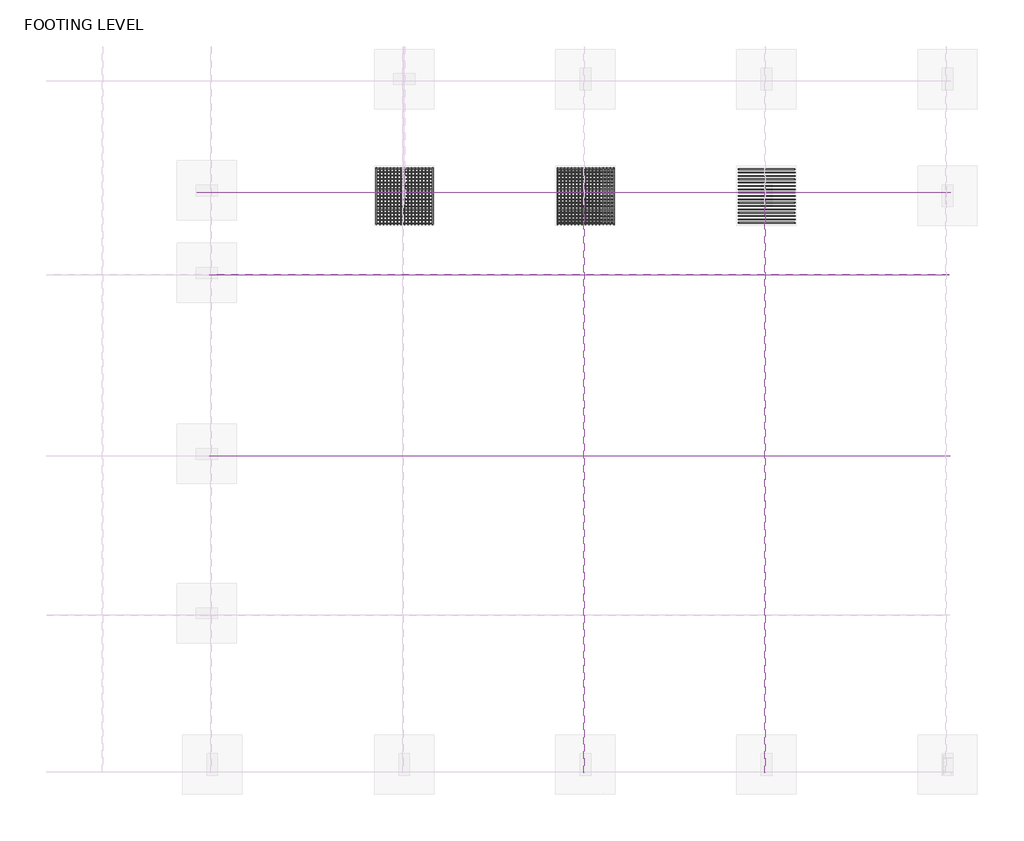
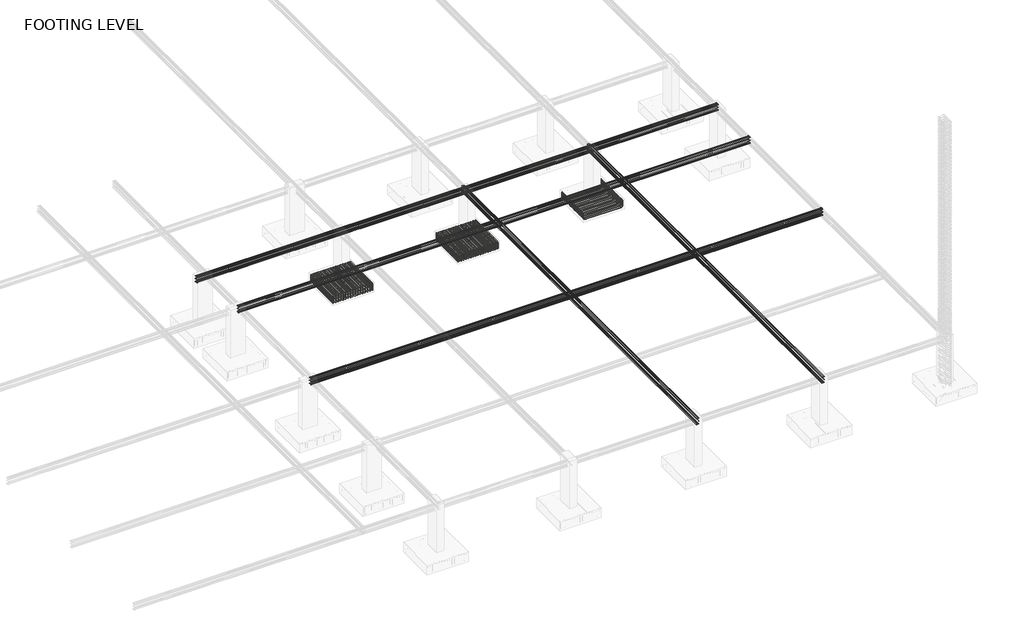
# One storey, part 8 of 19: 23 reinforcing bars.
"""IFC4 building model written with IfcOpenShell, lengths in millimetres."""

from ifc_helpers import new_model, si_unit, point, frame, origin, place, context, project, spatial, polyline, circle_curve, trimmed, segment, composite_curve, source, transform, mapped, element, save
from ifc_brep_helpers import swept_disk

model = new_model("IFC4")

# Units and contexts
model_context = context("Model", 3, world=origin())
ifc_project = project(units=[si_unit("LENGTHUNIT", "METRE", prefix="MILLI")], contexts=[model_context])

# Site, building, storey
site = spatial("IfcSite", under=ifc_project)
building = spatial("IfcBuilding", under=site)
storey = spatial("IfcBuildingStorey", under=building, Name="FOOTING LEVEL", Elevation=-3048.0)

# Reinforcing bars
placement = place(None, origin())
reinforcing_bar_shape = source(origin(), model_context, "Body", "SolidModel", [
    swept_disk(composite_curve([segment(polyline([(10639.8587563, -2750.5596072, -3548.0), (10639.8587563, -2750.5596072, -3225.9)]), True, "CONTINUOUS"), segment(trimmed(circle_curve(frame((10549.6587563, -2750.5596072, -3225.9), z_axis=(0.0, -1.0, 0.0), x_axis=(90.20000000000073, 0.0, 0.0)), 90.2), [point((10639.8587563, -2750.5596072, -3225.9))], [point((10549.6587563, -2750.5596072, -3135.7))], True, "CARTESIAN"), True, "CONTINUOUS"), segment(polyline([(10549.6587563, -2750.5596072, -3135.7), (8355.4587563, -2750.5596072, -3135.7)]), True, "CONTINUOUS"), segment(trimmed(circle_curve(frame((8355.4587563, -2750.5596072, -3225.9), z_axis=(0.0, -1.0, 0.0), x_axis=(0.0, 0.0, 90.20000000000027)), 90.2), [point((8355.4587563, -2750.5596072, -3135.7))], [point((8265.2587563, -2750.5596072, -3225.9))], True, "CARTESIAN"), True, "CONTINUOUS"), segment(polyline([(8265.2587563, -2750.5596072, -3225.9), (8265.2587563, -2750.5596072, -3548.0)]), True, "CONTINUOUS")], self_intersect=False), 12.7),
])
element("IfcReinforcingBar", 1, at=placement, inside=storey, context=model_context, shape_type="MappedRepresentation", body=[
    mapped(reinforcing_bar_shape, transform((0.0, 0.0, 0.0), x_axis=(1.0, 0.0, 0.0), y_axis=(0.0, 1.0, 0.0), z_axis=(0.0, 0.0, 1.0))),
    mapped(reinforcing_bar_shape, transform((0.0, -143.8496077, 0.0), x_axis=(1.0, 0.0, 0.0), y_axis=(0.0, 1.0, 0.0), z_axis=(0.0, 0.0, 1.0))),
    mapped(reinforcing_bar_shape, transform((0.0, -287.6992155, 0.0), x_axis=(1.0, 0.0, 0.0), y_axis=(0.0, 1.0, 0.0), z_axis=(0.0, 0.0, 1.0))),
    mapped(reinforcing_bar_shape, transform((0.0, -431.5488232, 0.0), x_axis=(1.0, 0.0, 0.0), y_axis=(0.0, 1.0, 0.0), z_axis=(0.0, 0.0, 1.0))),
    mapped(reinforcing_bar_shape, transform((0.0, -575.398431, 0.0), x_axis=(1.0, 0.0, 0.0), y_axis=(0.0, 1.0, 0.0), z_axis=(0.0, 0.0, 1.0))),
    mapped(reinforcing_bar_shape, transform((0.0, -719.2480387, 0.0), x_axis=(1.0, 0.0, 0.0), y_axis=(0.0, 1.0, 0.0), z_axis=(0.0, 0.0, 1.0))),
    mapped(reinforcing_bar_shape, transform((0.0, -863.0976465, 0.0), x_axis=(1.0, 0.0, 0.0), y_axis=(0.0, 1.0, 0.0), z_axis=(0.0, 0.0, 1.0))),
    mapped(reinforcing_bar_shape, transform((0.0, -1006.9472542, 0.0), x_axis=(1.0, 0.0, 0.0), y_axis=(0.0, 1.0, 0.0), z_axis=(0.0, 0.0, 1.0))),
    mapped(reinforcing_bar_shape, transform((0.0, -1150.796862, 0.0), x_axis=(1.0, 0.0, 0.0), y_axis=(0.0, 1.0, 0.0), z_axis=(0.0, 0.0, 1.0))),
    mapped(reinforcing_bar_shape, transform((0.0, -1294.6464697, 0.0), x_axis=(1.0, 0.0, 0.0), y_axis=(0.0, 1.0, 0.0), z_axis=(0.0, 0.0, 1.0))),
    mapped(reinforcing_bar_shape, transform((0.0, -1438.4960775, 0.0), x_axis=(1.0, 0.0, 0.0), y_axis=(0.0, 1.0, 0.0), z_axis=(0.0, 0.0, 1.0))),
    mapped(reinforcing_bar_shape, transform((0.0, -1582.3456852, 0.0), x_axis=(1.0, 0.0, 0.0), y_axis=(0.0, 1.0, 0.0), z_axis=(0.0, 0.0, 1.0))),
    mapped(reinforcing_bar_shape, transform((0.0, -1726.195293, 0.0), x_axis=(1.0, 0.0, 0.0), y_axis=(0.0, 1.0, 0.0), z_axis=(0.0, 0.0, 1.0))),
    mapped(reinforcing_bar_shape, transform((0.0, -1870.0449007, 0.0), x_axis=(1.0, 0.0, 0.0), y_axis=(0.0, 1.0, 0.0), z_axis=(0.0, 0.0, 1.0))),
    mapped(reinforcing_bar_shape, transform((0.0, -2013.8945085, 0.0), x_axis=(1.0, 0.0, 0.0), y_axis=(0.0, 1.0, 0.0), z_axis=(0.0, 0.0, 1.0))),
    mapped(reinforcing_bar_shape, transform((0.0, -2157.7441162, 0.0), x_axis=(1.0, 0.0, 0.0), y_axis=(0.0, 1.0, 0.0), z_axis=(0.0, 0.0, 1.0))),
    mapped(reinforcing_bar_shape, transform((0.0, -2301.5937239, 0.0), x_axis=(1.0, 0.0, 0.0), y_axis=(0.0, 1.0, 0.0), z_axis=(0.0, 0.0, 1.0))),
])
reinforcing_bar_2_shape = source(origin(), model_context, "Body", "SolidModel", [
    swept_disk(composite_curve([segment(polyline([(8265.2587563, -5091.5205555, -3173.0), (8265.2587563, -5091.5205555, -3495.1)]), True, "CONTINUOUS"), segment(trimmed(circle_curve(frame((8265.2587563, -5001.3205555, -3495.1), z_axis=(1.0, 0.0, 0.0), x_axis=(0.0, -90.19999999999982, 0.0)), 90.2), [point((8265.2587563, -5091.5205555, -3495.1))], [point((8265.2587563, -5001.3205555, -3585.3))], True, "CARTESIAN"), True, "CONTINUOUS"), segment(polyline([(8265.2587563, -5001.3205555, -3585.3), (8265.2587563, -2807.1205555, -3585.3)]), True, "CONTINUOUS"), segment(trimmed(circle_curve(frame((8265.2587563, -2807.1205555, -3495.1), z_axis=(1.0, 0.0, 0.0), x_axis=(0.0, 0.0, -90.20000000000027)), 90.2), [point((8265.2587563, -2807.1205555, -3585.3))], [point((8265.2587563, -2716.9205555, -3495.1))], True, "CARTESIAN"), True, "CONTINUOUS"), segment(polyline([(8265.2587563, -2716.9205555, -3495.1), (8265.2587563, -2716.9205555, -3173.0)]), True, "CONTINUOUS")], self_intersect=False), 12.7),
])
element("IfcReinforcingBar", 2, at=placement, inside=storey, context=model_context, shape_type="MappedRepresentation", body=[
    mapped(reinforcing_bar_2_shape, transform((0.0, 0.0, 0.0), x_axis=(1.0, 0.0, 0.0), y_axis=(0.0, 1.0, 0.0), z_axis=(0.0, 0.0, 1.0))),
    mapped(reinforcing_bar_2_shape, transform((148.4125, 0.0, 0.0), x_axis=(1.0, 0.0, 0.0), y_axis=(0.0, 1.0, 0.0), z_axis=(0.0, 0.0, 1.0))),
    mapped(reinforcing_bar_2_shape, transform((296.825, 0.0, 0.0), x_axis=(1.0, 0.0, 0.0), y_axis=(0.0, 1.0, 0.0), z_axis=(0.0, 0.0, 1.0))),
    mapped(reinforcing_bar_2_shape, transform((445.2375, 0.0, 0.0), x_axis=(1.0, 0.0, 0.0), y_axis=(0.0, 1.0, 0.0), z_axis=(0.0, 0.0, 1.0))),
    mapped(reinforcing_bar_2_shape, transform((593.65, 0.0, 0.0), x_axis=(1.0, 0.0, 0.0), y_axis=(0.0, 1.0, 0.0), z_axis=(0.0, 0.0, 1.0))),
    mapped(reinforcing_bar_2_shape, transform((742.0625, 0.0, 0.0), x_axis=(1.0, 0.0, 0.0), y_axis=(0.0, 1.0, 0.0), z_axis=(0.0, 0.0, 1.0))),
    mapped(reinforcing_bar_2_shape, transform((890.475, 0.0, 0.0), x_axis=(1.0, 0.0, 0.0), y_axis=(0.0, 1.0, 0.0), z_axis=(0.0, 0.0, 1.0))),
    mapped(reinforcing_bar_2_shape, transform((1038.8875, 0.0, 0.0), x_axis=(1.0, 0.0, 0.0), y_axis=(0.0, 1.0, 0.0), z_axis=(0.0, 0.0, 1.0))),
    mapped(reinforcing_bar_2_shape, transform((1187.3, 0.0, 0.0), x_axis=(1.0, 0.0, 0.0), y_axis=(0.0, 1.0, 0.0), z_axis=(0.0, 0.0, 1.0))),
    mapped(reinforcing_bar_2_shape, transform((1335.7125, 0.0, 0.0), x_axis=(1.0, 0.0, 0.0), y_axis=(0.0, 1.0, 0.0), z_axis=(0.0, 0.0, 1.0))),
    mapped(reinforcing_bar_2_shape, transform((1484.125, 0.0, 0.0), x_axis=(1.0, 0.0, 0.0), y_axis=(0.0, 1.0, 0.0), z_axis=(0.0, 0.0, 1.0))),
    mapped(reinforcing_bar_2_shape, transform((1632.5375, 0.0, 0.0), x_axis=(1.0, 0.0, 0.0), y_axis=(0.0, 1.0, 0.0), z_axis=(0.0, 0.0, 1.0))),
    mapped(reinforcing_bar_2_shape, transform((1780.95, 0.0, 0.0), x_axis=(1.0, 0.0, 0.0), y_axis=(0.0, 1.0, 0.0), z_axis=(0.0, 0.0, 1.0))),
    mapped(reinforcing_bar_2_shape, transform((1929.3625, 0.0, 0.0), x_axis=(1.0, 0.0, 0.0), y_axis=(0.0, 1.0, 0.0), z_axis=(0.0, 0.0, 1.0))),
    mapped(reinforcing_bar_2_shape, transform((2077.775, 0.0, 0.0), x_axis=(1.0, 0.0, 0.0), y_axis=(0.0, 1.0, 0.0), z_axis=(0.0, 0.0, 1.0))),
    mapped(reinforcing_bar_2_shape, transform((2226.1875, 0.0, 0.0), x_axis=(1.0, 0.0, 0.0), y_axis=(0.0, 1.0, 0.0), z_axis=(0.0, 0.0, 1.0))),
    mapped(reinforcing_bar_2_shape, transform((2374.6, 0.0, 0.0), x_axis=(1.0, 0.0, 0.0), y_axis=(0.0, 1.0, 0.0), z_axis=(0.0, 0.0, 1.0))),
])
reinforcing_bar_3_shape = source(origin(), model_context, "Body", "SolidModel", [
    swept_disk(composite_curve([segment(polyline([(8265.2587563, -2716.9205555, -3523.0), (8265.2587563, -2716.9205555, -3200.9)]), True, "CONTINUOUS"), segment(trimmed(circle_curve(frame((8265.2587563, -2807.1205555, -3200.9), z_axis=(1.0, 0.0, 0.0), x_axis=(0.0, 90.20000000000027, 0.0)), 90.2), [point((8265.2587563, -2716.9205555, -3200.9))], [point((8265.2587563, -2807.1205555, -3110.7))], True, "CARTESIAN"), True, "CONTINUOUS"), segment(polyline([(8265.2587563, -2807.1205555, -3110.7), (8265.2587563, -5001.3205555, -3110.7)]), True, "CONTINUOUS"), segment(trimmed(circle_curve(frame((8265.2587563, -5001.3205555, -3200.9), z_axis=(1.0, 0.0, 0.0), x_axis=(0.0, 0.0, 90.20000000000027)), 90.2), [point((8265.2587563, -5001.3205555, -3110.7))], [point((8265.2587563, -5091.5205555, -3200.9))], True, "CARTESIAN"), True, "CONTINUOUS"), segment(polyline([(8265.2587563, -5091.5205555, -3200.9), (8265.2587563, -5091.5205555, -3523.0)]), True, "CONTINUOUS")], self_intersect=False), 12.7),
])
element("IfcReinforcingBar", 3, at=placement, inside=storey, context=model_context, shape_type="MappedRepresentation", body=[
    mapped(reinforcing_bar_3_shape, transform((0.0, 0.0, 0.0), x_axis=(1.0, 0.0, 0.0), y_axis=(0.0, 1.0, 0.0), z_axis=(0.0, 0.0, 1.0))),
    mapped(reinforcing_bar_3_shape, transform((148.4125, 0.0, 0.0), x_axis=(1.0, 0.0, 0.0), y_axis=(0.0, 1.0, 0.0), z_axis=(0.0, 0.0, 1.0))),
    mapped(reinforcing_bar_3_shape, transform((296.825, 0.0, 0.0), x_axis=(1.0, 0.0, 0.0), y_axis=(0.0, 1.0, 0.0), z_axis=(0.0, 0.0, 1.0))),
    mapped(reinforcing_bar_3_shape, transform((445.2375, 0.0, 0.0), x_axis=(1.0, 0.0, 0.0), y_axis=(0.0, 1.0, 0.0), z_axis=(0.0, 0.0, 1.0))),
    mapped(reinforcing_bar_3_shape, transform((593.65, 0.0, 0.0), x_axis=(1.0, 0.0, 0.0), y_axis=(0.0, 1.0, 0.0), z_axis=(0.0, 0.0, 1.0))),
    mapped(reinforcing_bar_3_shape, transform((742.0625, 0.0, 0.0), x_axis=(1.0, 0.0, 0.0), y_axis=(0.0, 1.0, 0.0), z_axis=(0.0, 0.0, 1.0))),
    mapped(reinforcing_bar_3_shape, transform((890.475, 0.0, 0.0), x_axis=(1.0, 0.0, 0.0), y_axis=(0.0, 1.0, 0.0), z_axis=(0.0, 0.0, 1.0))),
    mapped(reinforcing_bar_3_shape, transform((1038.8875, 0.0, 0.0), x_axis=(1.0, 0.0, 0.0), y_axis=(0.0, 1.0, 0.0), z_axis=(0.0, 0.0, 1.0))),
    mapped(reinforcing_bar_3_shape, transform((1187.3, 0.0, 0.0), x_axis=(1.0, 0.0, 0.0), y_axis=(0.0, 1.0, 0.0), z_axis=(0.0, 0.0, 1.0))),
    mapped(reinforcing_bar_3_shape, transform((1335.7125, 0.0, 0.0), x_axis=(1.0, 0.0, 0.0), y_axis=(0.0, 1.0, 0.0), z_axis=(0.0, 0.0, 1.0))),
    mapped(reinforcing_bar_3_shape, transform((1484.125, 0.0, 0.0), x_axis=(1.0, 0.0, 0.0), y_axis=(0.0, 1.0, 0.0), z_axis=(0.0, 0.0, 1.0))),
    mapped(reinforcing_bar_3_shape, transform((1632.5375, 0.0, 0.0), x_axis=(1.0, 0.0, 0.0), y_axis=(0.0, 1.0, 0.0), z_axis=(0.0, 0.0, 1.0))),
    mapped(reinforcing_bar_3_shape, transform((1780.95, 0.0, 0.0), x_axis=(1.0, 0.0, 0.0), y_axis=(0.0, 1.0, 0.0), z_axis=(0.0, 0.0, 1.0))),
    mapped(reinforcing_bar_3_shape, transform((1929.3625, 0.0, 0.0), x_axis=(1.0, 0.0, 0.0), y_axis=(0.0, 1.0, 0.0), z_axis=(0.0, 0.0, 1.0))),
    mapped(reinforcing_bar_3_shape, transform((2077.775, 0.0, 0.0), x_axis=(1.0, 0.0, 0.0), y_axis=(0.0, 1.0, 0.0), z_axis=(0.0, 0.0, 1.0))),
    mapped(reinforcing_bar_3_shape, transform((2226.1875, 0.0, 0.0), x_axis=(1.0, 0.0, 0.0), y_axis=(0.0, 1.0, 0.0), z_axis=(0.0, 0.0, 1.0))),
    mapped(reinforcing_bar_3_shape, transform((2374.6, 0.0, 0.0), x_axis=(1.0, 0.0, 0.0), y_axis=(0.0, 1.0, 0.0), z_axis=(0.0, 0.0, 1.0))),
])
reinforcing_bar_4_shape = source(origin(), model_context, "Body", "SolidModel", [
    swept_disk(composite_curve([segment(polyline([(18259.8587563, -5025.9516566, -3148.0), (18259.8587563, -5025.9516566, -3470.1)]), True, "CONTINUOUS"), segment(trimmed(circle_curve(frame((18169.6587563, -5025.9516566, -3470.1), z_axis=(0.0, 1.0, 0.0), x_axis=(90.20000000000073, 0.0, 0.0)), 90.2), [point((18259.8587563, -5025.9516566, -3470.1))], [point((18169.6587563, -5025.9516566, -3560.3))], True, "CARTESIAN"), True, "CONTINUOUS"), segment(polyline([(18169.6587563, -5025.9516566, -3560.3), (15975.4587563, -5025.9516566, -3560.3)]), True, "CONTINUOUS"), segment(trimmed(circle_curve(frame((15975.4587563, -5025.9516566, -3470.1), z_axis=(0.0, 1.0, 0.0), x_axis=(0.0, 0.0, -90.20000000000027)), 90.2), [point((15975.4587563, -5025.9516566, -3560.3))], [point((15885.2587563, -5025.9516566, -3470.1))], True, "CARTESIAN"), True, "CONTINUOUS"), segment(polyline([(15885.2587563, -5025.9516566, -3470.1), (15885.2587563, -5025.9516566, -3148.0)]), True, "CONTINUOUS")], self_intersect=False), 12.7),
])
element("IfcReinforcingBar", 4, at=placement, inside=storey, context=model_context, shape_type="MappedRepresentation", body=[
    mapped(reinforcing_bar_4_shape, transform((0.0, 0.0, 0.0), x_axis=(1.0, 0.0, 0.0), y_axis=(0.0, 1.0, 0.0), z_axis=(0.0, 0.0, 1.0))),
    mapped(reinforcing_bar_4_shape, transform((0.0, 140.8090411, 0.0), x_axis=(1.0, 0.0, 0.0), y_axis=(0.0, 1.0, 0.0), z_axis=(0.0, 0.0, 1.0))),
    mapped(reinforcing_bar_4_shape, transform((0.0, 281.6180821, 0.0), x_axis=(1.0, 0.0, 0.0), y_axis=(0.0, 1.0, 0.0), z_axis=(0.0, 0.0, 1.0))),
    mapped(reinforcing_bar_4_shape, transform((0.0, 422.4271232, 0.0), x_axis=(1.0, 0.0, 0.0), y_axis=(0.0, 1.0, 0.0), z_axis=(0.0, 0.0, 1.0))),
    mapped(reinforcing_bar_4_shape, transform((0.0, 563.2361643, 0.0), x_axis=(1.0, 0.0, 0.0), y_axis=(0.0, 1.0, 0.0), z_axis=(0.0, 0.0, 1.0))),
    mapped(reinforcing_bar_4_shape, transform((0.0, 704.0452054, 0.0), x_axis=(1.0, 0.0, 0.0), y_axis=(0.0, 1.0, 0.0), z_axis=(0.0, 0.0, 1.0))),
    mapped(reinforcing_bar_4_shape, transform((0.0, 844.8542464, 0.0), x_axis=(1.0, 0.0, 0.0), y_axis=(0.0, 1.0, 0.0), z_axis=(0.0, 0.0, 1.0))),
    mapped(reinforcing_bar_4_shape, transform((0.0, 985.6632875, 0.0), x_axis=(1.0, 0.0, 0.0), y_axis=(0.0, 1.0, 0.0), z_axis=(0.0, 0.0, 1.0))),
    mapped(reinforcing_bar_4_shape, transform((0.0, 1126.4723286, 0.0), x_axis=(1.0, 0.0, 0.0), y_axis=(0.0, 1.0, 0.0), z_axis=(0.0, 0.0, 1.0))),
    mapped(reinforcing_bar_4_shape, transform((0.0, 1267.2813697, 0.0), x_axis=(1.0, 0.0, 0.0), y_axis=(0.0, 1.0, 0.0), z_axis=(0.0, 0.0, 1.0))),
    mapped(reinforcing_bar_4_shape, transform((0.0, 1408.0904107, 0.0), x_axis=(1.0, 0.0, 0.0), y_axis=(0.0, 1.0, 0.0), z_axis=(0.0, 0.0, 1.0))),
    mapped(reinforcing_bar_4_shape, transform((0.0, 1548.8994518, 0.0), x_axis=(1.0, 0.0, 0.0), y_axis=(0.0, 1.0, 0.0), z_axis=(0.0, 0.0, 1.0))),
    mapped(reinforcing_bar_4_shape, transform((0.0, 1689.7084929, 0.0), x_axis=(1.0, 0.0, 0.0), y_axis=(0.0, 1.0, 0.0), z_axis=(0.0, 0.0, 1.0))),
    mapped(reinforcing_bar_4_shape, transform((0.0, 1830.517534, 0.0), x_axis=(1.0, 0.0, 0.0), y_axis=(0.0, 1.0, 0.0), z_axis=(0.0, 0.0, 1.0))),
    mapped(reinforcing_bar_4_shape, transform((0.0, 1971.326575, 0.0), x_axis=(1.0, 0.0, 0.0), y_axis=(0.0, 1.0, 0.0), z_axis=(0.0, 0.0, 1.0))),
    mapped(reinforcing_bar_4_shape, transform((0.0, 2112.1356161, 0.0), x_axis=(1.0, 0.0, 0.0), y_axis=(0.0, 1.0, 0.0), z_axis=(0.0, 0.0, 1.0))),
    mapped(reinforcing_bar_4_shape, transform((0.0, 2252.9446572, 0.0), x_axis=(1.0, 0.0, 0.0), y_axis=(0.0, 1.0, 0.0), z_axis=(0.0, 0.0, 1.0))),
])
reinforcing_bar_5_shape = source(origin(), model_context, "Body", "SolidModel", [
    swept_disk(composite_curve([segment(polyline([(18259.8587563, -2750.5596072, -3548.0), (18259.8587563, -2750.5596072, -3225.9)]), True, "CONTINUOUS"), segment(trimmed(circle_curve(frame((18169.6587563, -2750.5596072, -3225.9), z_axis=(0.0, -1.0, 0.0), x_axis=(90.20000000000073, 0.0, 0.0)), 90.2), [point((18259.8587563, -2750.5596072, -3225.9))], [point((18169.6587563, -2750.5596072, -3135.7))], True, "CARTESIAN"), True, "CONTINUOUS"), segment(polyline([(18169.6587563, -2750.5596072, -3135.7), (15975.4587563, -2750.5596072, -3135.7)]), True, "CONTINUOUS"), segment(trimmed(circle_curve(frame((15975.4587563, -2750.5596072, -3225.9), z_axis=(0.0, -1.0, 0.0), x_axis=(0.0, 0.0, 90.20000000000027)), 90.2), [point((15975.4587563, -2750.5596072, -3135.7))], [point((15885.2587563, -2750.5596072, -3225.9))], True, "CARTESIAN"), True, "CONTINUOUS"), segment(polyline([(15885.2587563, -2750.5596072, -3225.9), (15885.2587563, -2750.5596072, -3548.0)]), True, "CONTINUOUS")], self_intersect=False), 12.7),
])
element("IfcReinforcingBar", 5, at=placement, inside=storey, context=model_context, shape_type="MappedRepresentation", body=[
    mapped(reinforcing_bar_5_shape, transform((0.0, 0.0, 0.0), x_axis=(1.0, 0.0, 0.0), y_axis=(0.0, 1.0, 0.0), z_axis=(0.0, 0.0, 1.0))),
    mapped(reinforcing_bar_5_shape, transform((0.0, -143.8496077, 0.0), x_axis=(1.0, 0.0, 0.0), y_axis=(0.0, 1.0, 0.0), z_axis=(0.0, 0.0, 1.0))),
    mapped(reinforcing_bar_5_shape, transform((0.0, -287.6992155, 0.0), x_axis=(1.0, 0.0, 0.0), y_axis=(0.0, 1.0, 0.0), z_axis=(0.0, 0.0, 1.0))),
    mapped(reinforcing_bar_5_shape, transform((0.0, -431.5488232, 0.0), x_axis=(1.0, 0.0, 0.0), y_axis=(0.0, 1.0, 0.0), z_axis=(0.0, 0.0, 1.0))),
    mapped(reinforcing_bar_5_shape, transform((0.0, -575.398431, 0.0), x_axis=(1.0, 0.0, 0.0), y_axis=(0.0, 1.0, 0.0), z_axis=(0.0, 0.0, 1.0))),
    mapped(reinforcing_bar_5_shape, transform((0.0, -719.2480387, 0.0), x_axis=(1.0, 0.0, 0.0), y_axis=(0.0, 1.0, 0.0), z_axis=(0.0, 0.0, 1.0))),
    mapped(reinforcing_bar_5_shape, transform((0.0, -863.0976465, 0.0), x_axis=(1.0, 0.0, 0.0), y_axis=(0.0, 1.0, 0.0), z_axis=(0.0, 0.0, 1.0))),
    mapped(reinforcing_bar_5_shape, transform((0.0, -1006.9472542, 0.0), x_axis=(1.0, 0.0, 0.0), y_axis=(0.0, 1.0, 0.0), z_axis=(0.0, 0.0, 1.0))),
    mapped(reinforcing_bar_5_shape, transform((0.0, -1150.796862, 0.0), x_axis=(1.0, 0.0, 0.0), y_axis=(0.0, 1.0, 0.0), z_axis=(0.0, 0.0, 1.0))),
    mapped(reinforcing_bar_5_shape, transform((0.0, -1294.6464697, 0.0), x_axis=(1.0, 0.0, 0.0), y_axis=(0.0, 1.0, 0.0), z_axis=(0.0, 0.0, 1.0))),
    mapped(reinforcing_bar_5_shape, transform((0.0, -1438.4960775, 0.0), x_axis=(1.0, 0.0, 0.0), y_axis=(0.0, 1.0, 0.0), z_axis=(0.0, 0.0, 1.0))),
    mapped(reinforcing_bar_5_shape, transform((0.0, -1582.3456852, 0.0), x_axis=(1.0, 0.0, 0.0), y_axis=(0.0, 1.0, 0.0), z_axis=(0.0, 0.0, 1.0))),
    mapped(reinforcing_bar_5_shape, transform((0.0, -1726.195293, 0.0), x_axis=(1.0, 0.0, 0.0), y_axis=(0.0, 1.0, 0.0), z_axis=(0.0, 0.0, 1.0))),
    mapped(reinforcing_bar_5_shape, transform((0.0, -1870.0449007, 0.0), x_axis=(1.0, 0.0, 0.0), y_axis=(0.0, 1.0, 0.0), z_axis=(0.0, 0.0, 1.0))),
    mapped(reinforcing_bar_5_shape, transform((0.0, -2013.8945085, 0.0), x_axis=(1.0, 0.0, 0.0), y_axis=(0.0, 1.0, 0.0), z_axis=(0.0, 0.0, 1.0))),
    mapped(reinforcing_bar_5_shape, transform((0.0, -2157.7441162, 0.0), x_axis=(1.0, 0.0, 0.0), y_axis=(0.0, 1.0, 0.0), z_axis=(0.0, 0.0, 1.0))),
    mapped(reinforcing_bar_5_shape, transform((0.0, -2301.5937239, 0.0), x_axis=(1.0, 0.0, 0.0), y_axis=(0.0, 1.0, 0.0), z_axis=(0.0, 0.0, 1.0))),
])
reinforcing_bar_6_shape = source(origin(), model_context, "Body", "SolidModel", [
    swept_disk(composite_curve([segment(polyline([(15885.2587563, -5091.5205555, -3173.0), (15885.2587563, -5091.5205555, -3495.1)]), True, "CONTINUOUS"), segment(trimmed(circle_curve(frame((15885.2587563, -5001.3205555, -3495.1), z_axis=(1.0, 0.0, 0.0), x_axis=(0.0, -90.19999999999982, 0.0)), 90.2), [point((15885.2587563, -5091.5205555, -3495.1))], [point((15885.2587563, -5001.3205555, -3585.3))], True, "CARTESIAN"), True, "CONTINUOUS"), segment(polyline([(15885.2587563, -5001.3205555, -3585.3), (15885.2587563, -2807.1205555, -3585.3)]), True, "CONTINUOUS"), segment(trimmed(circle_curve(frame((15885.2587563, -2807.1205555, -3495.1), z_axis=(1.0, 0.0, 0.0), x_axis=(0.0, 0.0, -90.20000000000027)), 90.2), [point((15885.2587563, -2807.1205555, -3585.3))], [point((15885.2587563, -2716.9205555, -3495.1))], True, "CARTESIAN"), True, "CONTINUOUS"), segment(polyline([(15885.2587563, -2716.9205555, -3495.1), (15885.2587563, -2716.9205555, -3173.0)]), True, "CONTINUOUS")], self_intersect=False), 12.7),
])
element("IfcReinforcingBar", 6, at=placement, inside=storey, context=model_context, shape_type="MappedRepresentation", body=[
    mapped(reinforcing_bar_6_shape, transform((0.0, 0.0, 0.0), x_axis=(1.0, 0.0, 0.0), y_axis=(0.0, 1.0, 0.0), z_axis=(0.0, 0.0, 1.0))),
    mapped(reinforcing_bar_6_shape, transform((148.4125, 0.0, 0.0), x_axis=(1.0, 0.0, 0.0), y_axis=(0.0, 1.0, 0.0), z_axis=(0.0, 0.0, 1.0))),
    mapped(reinforcing_bar_6_shape, transform((296.825, 0.0, 0.0), x_axis=(1.0, 0.0, 0.0), y_axis=(0.0, 1.0, 0.0), z_axis=(0.0, 0.0, 1.0))),
    mapped(reinforcing_bar_6_shape, transform((445.2375, 0.0, 0.0), x_axis=(1.0, 0.0, 0.0), y_axis=(0.0, 1.0, 0.0), z_axis=(0.0, 0.0, 1.0))),
    mapped(reinforcing_bar_6_shape, transform((593.65, 0.0, 0.0), x_axis=(1.0, 0.0, 0.0), y_axis=(0.0, 1.0, 0.0), z_axis=(0.0, 0.0, 1.0))),
    mapped(reinforcing_bar_6_shape, transform((742.0625, 0.0, 0.0), x_axis=(1.0, 0.0, 0.0), y_axis=(0.0, 1.0, 0.0), z_axis=(0.0, 0.0, 1.0))),
    mapped(reinforcing_bar_6_shape, transform((890.475, 0.0, 0.0), x_axis=(1.0, 0.0, 0.0), y_axis=(0.0, 1.0, 0.0), z_axis=(0.0, 0.0, 1.0))),
    mapped(reinforcing_bar_6_shape, transform((1038.8875, 0.0, 0.0), x_axis=(1.0, 0.0, 0.0), y_axis=(0.0, 1.0, 0.0), z_axis=(0.0, 0.0, 1.0))),
    mapped(reinforcing_bar_6_shape, transform((1187.3, 0.0, 0.0), x_axis=(1.0, 0.0, 0.0), y_axis=(0.0, 1.0, 0.0), z_axis=(0.0, 0.0, 1.0))),
    mapped(reinforcing_bar_6_shape, transform((1335.7125, 0.0, 0.0), x_axis=(1.0, 0.0, 0.0), y_axis=(0.0, 1.0, 0.0), z_axis=(0.0, 0.0, 1.0))),
    mapped(reinforcing_bar_6_shape, transform((1484.125, 0.0, 0.0), x_axis=(1.0, 0.0, 0.0), y_axis=(0.0, 1.0, 0.0), z_axis=(0.0, 0.0, 1.0))),
    mapped(reinforcing_bar_6_shape, transform((1632.5375, 0.0, 0.0), x_axis=(1.0, 0.0, 0.0), y_axis=(0.0, 1.0, 0.0), z_axis=(0.0, 0.0, 1.0))),
    mapped(reinforcing_bar_6_shape, transform((1780.95, 0.0, 0.0), x_axis=(1.0, 0.0, 0.0), y_axis=(0.0, 1.0, 0.0), z_axis=(0.0, 0.0, 1.0))),
    mapped(reinforcing_bar_6_shape, transform((1929.3625, 0.0, 0.0), x_axis=(1.0, 0.0, 0.0), y_axis=(0.0, 1.0, 0.0), z_axis=(0.0, 0.0, 1.0))),
    mapped(reinforcing_bar_6_shape, transform((2077.775, 0.0, 0.0), x_axis=(1.0, 0.0, 0.0), y_axis=(0.0, 1.0, 0.0), z_axis=(0.0, 0.0, 1.0))),
    mapped(reinforcing_bar_6_shape, transform((2226.1875, 0.0, 0.0), x_axis=(1.0, 0.0, 0.0), y_axis=(0.0, 1.0, 0.0), z_axis=(0.0, 0.0, 1.0))),
    mapped(reinforcing_bar_6_shape, transform((2374.6, 0.0, 0.0), x_axis=(1.0, 0.0, 0.0), y_axis=(0.0, 1.0, 0.0), z_axis=(0.0, 0.0, 1.0))),
])
reinforcing_bar_7_shape = source(origin(), model_context, "Body", "SolidModel", [
    swept_disk(composite_curve([segment(polyline([(15885.2587563, -2716.9205555, -3523.0), (15885.2587563, -2716.9205555, -3200.9)]), True, "CONTINUOUS"), segment(trimmed(circle_curve(frame((15885.2587563, -2807.1205555, -3200.9), z_axis=(1.0, 0.0, 0.0), x_axis=(0.0, 90.20000000000027, 0.0)), 90.2), [point((15885.2587563, -2716.9205555, -3200.9))], [point((15885.2587563, -2807.1205555, -3110.7))], True, "CARTESIAN"), True, "CONTINUOUS"), segment(polyline([(15885.2587563, -2807.1205555, -3110.7), (15885.2587563, -5001.3205555, -3110.7)]), True, "CONTINUOUS"), segment(trimmed(circle_curve(frame((15885.2587563, -5001.3205555, -3200.9), z_axis=(1.0, 0.0, 0.0), x_axis=(0.0, 0.0, 90.20000000000027)), 90.2), [point((15885.2587563, -5001.3205555, -3110.7))], [point((15885.2587563, -5091.5205555, -3200.9))], True, "CARTESIAN"), True, "CONTINUOUS"), segment(polyline([(15885.2587563, -5091.5205555, -3200.9), (15885.2587563, -5091.5205555, -3523.0)]), True, "CONTINUOUS")], self_intersect=False), 12.7),
])
element("IfcReinforcingBar", 7, at=placement, inside=storey, context=model_context, shape_type="MappedRepresentation", body=[
    mapped(reinforcing_bar_7_shape, transform((0.0, 0.0, 0.0), x_axis=(1.0, 0.0, 0.0), y_axis=(0.0, 1.0, 0.0), z_axis=(0.0, 0.0, 1.0))),
    mapped(reinforcing_bar_7_shape, transform((148.4125, 0.0, 0.0), x_axis=(1.0, 0.0, 0.0), y_axis=(0.0, 1.0, 0.0), z_axis=(0.0, 0.0, 1.0))),
    mapped(reinforcing_bar_7_shape, transform((296.825, 0.0, 0.0), x_axis=(1.0, 0.0, 0.0), y_axis=(0.0, 1.0, 0.0), z_axis=(0.0, 0.0, 1.0))),
    mapped(reinforcing_bar_7_shape, transform((445.2375, 0.0, 0.0), x_axis=(1.0, 0.0, 0.0), y_axis=(0.0, 1.0, 0.0), z_axis=(0.0, 0.0, 1.0))),
    mapped(reinforcing_bar_7_shape, transform((593.65, 0.0, 0.0), x_axis=(1.0, 0.0, 0.0), y_axis=(0.0, 1.0, 0.0), z_axis=(0.0, 0.0, 1.0))),
    mapped(reinforcing_bar_7_shape, transform((742.0625, 0.0, 0.0), x_axis=(1.0, 0.0, 0.0), y_axis=(0.0, 1.0, 0.0), z_axis=(0.0, 0.0, 1.0))),
    mapped(reinforcing_bar_7_shape, transform((890.475, 0.0, 0.0), x_axis=(1.0, 0.0, 0.0), y_axis=(0.0, 1.0, 0.0), z_axis=(0.0, 0.0, 1.0))),
    mapped(reinforcing_bar_7_shape, transform((1038.8875, 0.0, 0.0), x_axis=(1.0, 0.0, 0.0), y_axis=(0.0, 1.0, 0.0), z_axis=(0.0, 0.0, 1.0))),
    mapped(reinforcing_bar_7_shape, transform((1187.3, 0.0, 0.0), x_axis=(1.0, 0.0, 0.0), y_axis=(0.0, 1.0, 0.0), z_axis=(0.0, 0.0, 1.0))),
    mapped(reinforcing_bar_7_shape, transform((1335.7125, 0.0, 0.0), x_axis=(1.0, 0.0, 0.0), y_axis=(0.0, 1.0, 0.0), z_axis=(0.0, 0.0, 1.0))),
    mapped(reinforcing_bar_7_shape, transform((1484.125, 0.0, 0.0), x_axis=(1.0, 0.0, 0.0), y_axis=(0.0, 1.0, 0.0), z_axis=(0.0, 0.0, 1.0))),
    mapped(reinforcing_bar_7_shape, transform((1632.5375, 0.0, 0.0), x_axis=(1.0, 0.0, 0.0), y_axis=(0.0, 1.0, 0.0), z_axis=(0.0, 0.0, 1.0))),
    mapped(reinforcing_bar_7_shape, transform((1780.95, 0.0, 0.0), x_axis=(1.0, 0.0, 0.0), y_axis=(0.0, 1.0, 0.0), z_axis=(0.0, 0.0, 1.0))),
    mapped(reinforcing_bar_7_shape, transform((1929.3625, 0.0, 0.0), x_axis=(1.0, 0.0, 0.0), y_axis=(0.0, 1.0, 0.0), z_axis=(0.0, 0.0, 1.0))),
    mapped(reinforcing_bar_7_shape, transform((2077.775, 0.0, 0.0), x_axis=(1.0, 0.0, 0.0), y_axis=(0.0, 1.0, 0.0), z_axis=(0.0, 0.0, 1.0))),
    mapped(reinforcing_bar_7_shape, transform((2226.1875, 0.0, 0.0), x_axis=(1.0, 0.0, 0.0), y_axis=(0.0, 1.0, 0.0), z_axis=(0.0, 0.0, 1.0))),
    mapped(reinforcing_bar_7_shape, transform((2374.6, 0.0, 0.0), x_axis=(1.0, 0.0, 0.0), y_axis=(0.0, 1.0, 0.0), z_axis=(0.0, 0.0, 1.0))),
])
reinforcing_bar_8_shape = source(origin(), model_context, "Body", "SolidModel", [
    swept_disk(composite_curve([segment(polyline([(25879.8587563, -5025.9516566, -3148.0), (25879.8587563, -5025.9516566, -3470.1)]), True, "CONTINUOUS"), segment(trimmed(circle_curve(frame((25789.6587563, -5025.9516566, -3470.1), z_axis=(0.0, 1.0, 0.0), x_axis=(90.20000000000073, 0.0, 0.0)), 90.2), [point((25879.8587563, -5025.9516566, -3470.1))], [point((25789.6587563, -5025.9516566, -3560.3))], True, "CARTESIAN"), True, "CONTINUOUS"), segment(polyline([(25789.6587563, -5025.9516566, -3560.3), (23595.4587563, -5025.9516566, -3560.3)]), True, "CONTINUOUS"), segment(trimmed(circle_curve(frame((23595.4587563, -5025.9516566, -3470.1), z_axis=(0.0, 1.0, 0.0), x_axis=(0.0, 0.0, -90.20000000000027)), 90.2), [point((23595.4587563, -5025.9516566, -3560.3))], [point((23505.2587563, -5025.9516566, -3470.1))], True, "CARTESIAN"), True, "CONTINUOUS"), segment(polyline([(23505.2587563, -5025.9516566, -3470.1), (23505.2587563, -5025.9516566, -3148.0)]), True, "CONTINUOUS")], self_intersect=False), 12.7),
])
element("IfcReinforcingBar", 8, at=placement, inside=storey, context=model_context, shape_type="MappedRepresentation", body=[
    mapped(reinforcing_bar_8_shape, transform((0.0, 0.0, 0.0), x_axis=(1.0, 0.0, 0.0), y_axis=(0.0, 1.0, 0.0), z_axis=(0.0, 0.0, 1.0))),
    mapped(reinforcing_bar_8_shape, transform((0.0, 140.8090411, 0.0), x_axis=(1.0, 0.0, 0.0), y_axis=(0.0, 1.0, 0.0), z_axis=(0.0, 0.0, 1.0))),
    mapped(reinforcing_bar_8_shape, transform((0.0, 281.6180821, 0.0), x_axis=(1.0, 0.0, 0.0), y_axis=(0.0, 1.0, 0.0), z_axis=(0.0, 0.0, 1.0))),
    mapped(reinforcing_bar_8_shape, transform((0.0, 422.4271232, 0.0), x_axis=(1.0, 0.0, 0.0), y_axis=(0.0, 1.0, 0.0), z_axis=(0.0, 0.0, 1.0))),
    mapped(reinforcing_bar_8_shape, transform((0.0, 563.2361643, 0.0), x_axis=(1.0, 0.0, 0.0), y_axis=(0.0, 1.0, 0.0), z_axis=(0.0, 0.0, 1.0))),
    mapped(reinforcing_bar_8_shape, transform((0.0, 704.0452054, 0.0), x_axis=(1.0, 0.0, 0.0), y_axis=(0.0, 1.0, 0.0), z_axis=(0.0, 0.0, 1.0))),
    mapped(reinforcing_bar_8_shape, transform((0.0, 844.8542464, 0.0), x_axis=(1.0, 0.0, 0.0), y_axis=(0.0, 1.0, 0.0), z_axis=(0.0, 0.0, 1.0))),
    mapped(reinforcing_bar_8_shape, transform((0.0, 985.6632875, 0.0), x_axis=(1.0, 0.0, 0.0), y_axis=(0.0, 1.0, 0.0), z_axis=(0.0, 0.0, 1.0))),
    mapped(reinforcing_bar_8_shape, transform((0.0, 1126.4723286, 0.0), x_axis=(1.0, 0.0, 0.0), y_axis=(0.0, 1.0, 0.0), z_axis=(0.0, 0.0, 1.0))),
    mapped(reinforcing_bar_8_shape, transform((0.0, 1267.2813697, 0.0), x_axis=(1.0, 0.0, 0.0), y_axis=(0.0, 1.0, 0.0), z_axis=(0.0, 0.0, 1.0))),
    mapped(reinforcing_bar_8_shape, transform((0.0, 1408.0904107, 0.0), x_axis=(1.0, 0.0, 0.0), y_axis=(0.0, 1.0, 0.0), z_axis=(0.0, 0.0, 1.0))),
    mapped(reinforcing_bar_8_shape, transform((0.0, 1548.8994518, 0.0), x_axis=(1.0, 0.0, 0.0), y_axis=(0.0, 1.0, 0.0), z_axis=(0.0, 0.0, 1.0))),
    mapped(reinforcing_bar_8_shape, transform((0.0, 1689.7084929, 0.0), x_axis=(1.0, 0.0, 0.0), y_axis=(0.0, 1.0, 0.0), z_axis=(0.0, 0.0, 1.0))),
    mapped(reinforcing_bar_8_shape, transform((0.0, 1830.517534, 0.0), x_axis=(1.0, 0.0, 0.0), y_axis=(0.0, 1.0, 0.0), z_axis=(0.0, 0.0, 1.0))),
    mapped(reinforcing_bar_8_shape, transform((0.0, 1971.326575, 0.0), x_axis=(1.0, 0.0, 0.0), y_axis=(0.0, 1.0, 0.0), z_axis=(0.0, 0.0, 1.0))),
    mapped(reinforcing_bar_8_shape, transform((0.0, 2112.1356161, 0.0), x_axis=(1.0, 0.0, 0.0), y_axis=(0.0, 1.0, 0.0), z_axis=(0.0, 0.0, 1.0))),
    mapped(reinforcing_bar_8_shape, transform((0.0, 2252.9446572, 0.0), x_axis=(1.0, 0.0, 0.0), y_axis=(0.0, 1.0, 0.0), z_axis=(0.0, 0.0, 1.0))),
])
reinforcing_bar_9_shape = source(origin(), model_context, "Body", "SolidModel", [
    swept_disk(composite_curve([segment(polyline([(729.5587563, -3745.4411922, -412.7206367), (32427.6293504, -3745.4411922, -412.7206367)]), True, "CONTINUOUS")], self_intersect=False), 7.95),
])
element("IfcReinforcingBar", 9, at=placement, inside=storey, context=model_context, shape_type="MappedRepresentation", body=[
    mapped(reinforcing_bar_9_shape, transform((0.0, 0.0, 0.0), x_axis=(1.0, 0.0, 0.0), y_axis=(0.0, 1.0, 0.0), z_axis=(0.0, 0.0, 1.0))),
    mapped(reinforcing_bar_9_shape, transform((0.0, 69.8206367, 0.0), x_axis=(1.0, 0.0, 0.0), y_axis=(0.0, 1.0, 0.0), z_axis=(0.0, 0.0, 1.0))),
    mapped(reinforcing_bar_9_shape, transform((0.0, 139.6412734, 0.0), x_axis=(1.0, 0.0, 0.0), y_axis=(0.0, 1.0, 0.0), z_axis=(0.0, 0.0, 1.0))),
])
reinforcing_bar_10_shape = source(origin(), model_context, "Body", "SolidModel", [
    swept_disk(composite_curve([segment(polyline([(729.5587563, -3745.4411922, -44.4793633), (32423.5267568, -3745.4411922, -44.4793633)]), True, "CONTINUOUS")], self_intersect=False), 7.95),
])
element("IfcReinforcingBar", 10, at=placement, inside=storey, context=model_context, shape_type="MappedRepresentation", body=[
    mapped(reinforcing_bar_10_shape, transform((0.0, 0.0, 0.0), x_axis=(1.0, 0.0, 0.0), y_axis=(0.0, 1.0, 0.0), z_axis=(0.0, 0.0, 1.0))),
    mapped(reinforcing_bar_10_shape, transform((0.0, 69.8206367, 0.0), x_axis=(1.0, 0.0, 0.0), y_axis=(0.0, 1.0, 0.0), z_axis=(0.0, 0.0, 1.0))),
    mapped(reinforcing_bar_10_shape, transform((0.0, 139.6412734, 0.0), x_axis=(1.0, 0.0, 0.0), y_axis=(0.0, 1.0, 0.0), z_axis=(0.0, 0.0, 1.0))),
])
reinforcing_bar_11_shape = source(origin(), model_context, "Body", "SolidModel", [
    swept_disk(composite_curve([segment(polyline([(729.5587563, -3602.2705555, -228.3387181), (32423.0777485, -3602.2705555, -228.3387181)]), True, "CONTINUOUS")], self_intersect=False), 7.95),
])
element("IfcReinforcingBar", 11, at=placement, inside=storey, context=model_context, shape_type="MappedRepresentation", body=[
    mapped(reinforcing_bar_11_shape, transform((0.0, 0.0, 0.0), x_axis=(1.0, 0.0, 0.0), y_axis=(0.0, 1.0, 0.0), z_axis=(0.0, 0.0, 1.0))),
    mapped(reinforcing_bar_11_shape, transform((0.0, -146.7, 0.0), x_axis=(1.0, 0.0, 0.0), y_axis=(0.0, 1.0, 0.0), z_axis=(0.0, 0.0, 1.0))),
])
reinforcing_bar_12_shape = source(origin(), model_context, "Body", "SolidModel", [
    swept_disk(composite_curve([segment(polyline([(32380.5008534, -14692.8999188, -412.7206367), (1260.2881621, -14692.8999188, -412.7206367)]), True, "CONTINUOUS")], self_intersect=False), 7.95),
])
element("IfcReinforcingBar", 12, at=placement, inside=storey, context=model_context, shape_type="MappedRepresentation", body=[
    mapped(reinforcing_bar_12_shape, transform((0.0, 0.0, 0.0), x_axis=(1.0, 0.0, 0.0), y_axis=(0.0, 1.0, 0.0), z_axis=(0.0, 0.0, 1.0))),
    mapped(reinforcing_bar_12_shape, transform((0.0, -69.8206367, 0.0), x_axis=(1.0, 0.0, 0.0), y_axis=(0.0, 1.0, 0.0), z_axis=(0.0, 0.0, 1.0))),
    mapped(reinforcing_bar_12_shape, transform((0.0, -139.6412734, 0.0), x_axis=(1.0, 0.0, 0.0), y_axis=(0.0, 1.0, 0.0), z_axis=(0.0, 0.0, 1.0))),
])
reinforcing_bar_13_shape = source(origin(), model_context, "Body", "SolidModel", [
    swept_disk(composite_curve([segment(polyline([(32384.1053785, -14692.8999188, -44.4793633), (1264.3907557, -14692.8999188, -44.4793633)]), True, "CONTINUOUS")], self_intersect=False), 7.95),
])
element("IfcReinforcingBar", 13, at=placement, inside=storey, context=model_context, shape_type="MappedRepresentation", body=[
    mapped(reinforcing_bar_13_shape, transform((0.0, 0.0, 0.0), x_axis=(1.0, 0.0, 0.0), y_axis=(0.0, 1.0, 0.0), z_axis=(0.0, 0.0, 1.0))),
    mapped(reinforcing_bar_13_shape, transform((0.0, -69.8206367, 0.0), x_axis=(1.0, 0.0, 0.0), y_axis=(0.0, 1.0, 0.0), z_axis=(0.0, 0.0, 1.0))),
    mapped(reinforcing_bar_13_shape, transform((0.0, -139.6412734, 0.0), x_axis=(1.0, 0.0, 0.0), y_axis=(0.0, 1.0, 0.0), z_axis=(0.0, 0.0, 1.0))),
])
reinforcing_bar_14_shape = source(origin(), model_context, "Body", "SolidModel", [
    swept_disk(composite_curve([segment(polyline([(32390.4132976, -14836.0705555, -228.3387181), (1264.839764, -14836.0705555, -228.3387181)]), True, "CONTINUOUS")], self_intersect=False), 7.95),
])
element("IfcReinforcingBar", 14, at=placement, inside=storey, context=model_context, shape_type="MappedRepresentation", body=[
    mapped(reinforcing_bar_14_shape, transform((0.0, 0.0, 0.0), x_axis=(1.0, 0.0, 0.0), y_axis=(0.0, 1.0, 0.0), z_axis=(0.0, 0.0, 1.0))),
    mapped(reinforcing_bar_14_shape, transform((0.0, 146.7, 0.0), x_axis=(1.0, 0.0, 0.0), y_axis=(0.0, 1.0, 0.0), z_axis=(0.0, 0.0, 1.0))),
])
reinforcing_bar_15_shape = source(origin(), model_context, "Body", "SolidModel", [
    swept_disk(composite_curve([segment(polyline([(32370.593473, -7072.8999188, -412.7206367), (1260.2881621, -7072.8999188, -412.7206367)]), True, "CONTINUOUS")], self_intersect=False), 7.95),
])
element("IfcReinforcingBar", 15, at=placement, inside=storey, context=model_context, shape_type="MappedRepresentation", body=[
    mapped(reinforcing_bar_15_shape, transform((0.0, 0.0, 0.0), x_axis=(1.0, 0.0, 0.0), y_axis=(0.0, 1.0, 0.0), z_axis=(0.0, 0.0, 1.0))),
    mapped(reinforcing_bar_15_shape, transform((0.0, -69.8206367, 0.0), x_axis=(1.0, 0.0, 0.0), y_axis=(0.0, 1.0, 0.0), z_axis=(0.0, 0.0, 1.0))),
    mapped(reinforcing_bar_15_shape, transform((0.0, -139.6412734, 0.0), x_axis=(1.0, 0.0, 0.0), y_axis=(0.0, 1.0, 0.0), z_axis=(0.0, 0.0, 1.0))),
])
reinforcing_bar_16_shape = source(origin(), model_context, "Body", "SolidModel", [
    swept_disk(composite_curve([segment(polyline([(32374.7049972, -7072.8999188, -44.4793633), (1264.3907557, -7072.8999188, -44.4793633)]), True, "CONTINUOUS")], self_intersect=False), 7.95),
])
element("IfcReinforcingBar", 16, at=placement, inside=storey, context=model_context, shape_type="MappedRepresentation", body=[
    mapped(reinforcing_bar_16_shape, transform((0.0, 0.0, 0.0), x_axis=(1.0, 0.0, 0.0), y_axis=(0.0, 1.0, 0.0), z_axis=(0.0, 0.0, 1.0))),
    mapped(reinforcing_bar_16_shape, transform((0.0, -69.8206367, 0.0), x_axis=(1.0, 0.0, 0.0), y_axis=(0.0, 1.0, 0.0), z_axis=(0.0, 0.0, 1.0))),
    mapped(reinforcing_bar_16_shape, transform((0.0, -139.6412734, 0.0), x_axis=(1.0, 0.0, 0.0), y_axis=(0.0, 1.0, 0.0), z_axis=(0.0, 0.0, 1.0))),
])
reinforcing_bar_17_shape = source(origin(), model_context, "Body", "SolidModel", [
    swept_disk(composite_curve([segment(polyline([(32370.593473, -7216.0705555, -228.3387181), (1264.839764, -7216.0705555, -228.3387181)]), True, "CONTINUOUS")], self_intersect=False), 7.95),
])
element("IfcReinforcingBar", 17, at=placement, inside=storey, context=model_context, shape_type="MappedRepresentation", body=[
    mapped(reinforcing_bar_17_shape, transform((0.0, 0.0, 0.0), x_axis=(1.0, 0.0, 0.0), y_axis=(0.0, 1.0, 0.0), z_axis=(0.0, 0.0, 1.0))),
    mapped(reinforcing_bar_17_shape, transform((0.0, 146.7, 0.0), x_axis=(1.0, 0.0, 0.0), y_axis=(0.0, 1.0, 0.0), z_axis=(0.0, 0.0, 1.0))),
])
reinforcing_bar_18_shape = source(origin(), model_context, "Body", "SolidModel", [
    swept_disk(composite_curve([segment(polyline([(24622.7381195, -3487.0205555, -412.7206367), (24622.7381195, -28174.6911496, -412.7206367)]), True, "CONTINUOUS")], self_intersect=False), 7.95),
])
element("IfcReinforcingBar", 18, at=placement, inside=storey, context=model_context, shape_type="MappedRepresentation", body=[
    mapped(reinforcing_bar_18_shape, transform((0.0, 0.0, 0.0), x_axis=(1.0, 0.0, 0.0), y_axis=(0.0, 1.0, 0.0), z_axis=(0.0, 0.0, 1.0))),
    mapped(reinforcing_bar_18_shape, transform((69.8206367, 0.0, 0.0), x_axis=(1.0, 0.0, 0.0), y_axis=(0.0, 1.0, 0.0), z_axis=(0.0, 0.0, 1.0))),
    mapped(reinforcing_bar_18_shape, transform((139.6412734, 0.0, 0.0), x_axis=(1.0, 0.0, 0.0), y_axis=(0.0, 1.0, 0.0), z_axis=(0.0, 0.0, 1.0))),
])
reinforcing_bar_19_shape = source(origin(), model_context, "Body", "SolidModel", [
    swept_disk(composite_curve([segment(polyline([(24622.7381195, -3487.0205555, -44.4793633), (24622.7381195, -28170.588556, -44.4793633)]), True, "CONTINUOUS")], self_intersect=False), 7.95),
])
element("IfcReinforcingBar", 19, at=placement, inside=storey, context=model_context, shape_type="MappedRepresentation", body=[
    mapped(reinforcing_bar_19_shape, transform((0.0, 0.0, 0.0), x_axis=(1.0, 0.0, 0.0), y_axis=(0.0, 1.0, 0.0), z_axis=(0.0, 0.0, 1.0))),
    mapped(reinforcing_bar_19_shape, transform((69.8206367, 0.0, 0.0), x_axis=(1.0, 0.0, 0.0), y_axis=(0.0, 1.0, 0.0), z_axis=(0.0, 0.0, 1.0))),
    mapped(reinforcing_bar_19_shape, transform((139.6412734, 0.0, 0.0), x_axis=(1.0, 0.0, 0.0), y_axis=(0.0, 1.0, 0.0), z_axis=(0.0, 0.0, 1.0))),
])
reinforcing_bar_20_shape = source(origin(), model_context, "Body", "SolidModel", [
    swept_disk(composite_curve([segment(polyline([(24765.9087563, -3487.0205555, -228.3387181), (24765.9087563, -28170.1395477, -228.3387181)]), True, "CONTINUOUS")], self_intersect=False), 7.95),
])
element("IfcReinforcingBar", 20, at=placement, inside=storey, context=model_context, shape_type="MappedRepresentation", body=[
    mapped(reinforcing_bar_20_shape, transform((0.0, 0.0, 0.0), x_axis=(1.0, 0.0, 0.0), y_axis=(0.0, 1.0, 0.0), z_axis=(0.0, 0.0, 1.0))),
    mapped(reinforcing_bar_20_shape, transform((-146.7, 0.0, 0.0), x_axis=(1.0, 0.0, 0.0), y_axis=(0.0, 1.0, 0.0), z_axis=(0.0, 0.0, 1.0))),
])
reinforcing_bar_21_shape = source(origin(), model_context, "Body", "SolidModel", [
    swept_disk(composite_curve([segment(polyline([(17002.7381195, -3487.0205555, -412.7206367), (17002.7381195, -28174.6911496, -412.7206367)]), True, "CONTINUOUS")], self_intersect=False), 7.95),
])
element("IfcReinforcingBar", 21, at=placement, inside=storey, context=model_context, shape_type="MappedRepresentation", body=[
    mapped(reinforcing_bar_21_shape, transform((0.0, 0.0, 0.0), x_axis=(1.0, 0.0, 0.0), y_axis=(0.0, 1.0, 0.0), z_axis=(0.0, 0.0, 1.0))),
    mapped(reinforcing_bar_21_shape, transform((69.8206367, 0.0, 0.0), x_axis=(1.0, 0.0, 0.0), y_axis=(0.0, 1.0, 0.0), z_axis=(0.0, 0.0, 1.0))),
    mapped(reinforcing_bar_21_shape, transform((139.6412734, 0.0, 0.0), x_axis=(1.0, 0.0, 0.0), y_axis=(0.0, 1.0, 0.0), z_axis=(0.0, 0.0, 1.0))),
])
reinforcing_bar_22_shape = source(origin(), model_context, "Body", "SolidModel", [
    swept_disk(composite_curve([segment(polyline([(17002.7381195, -3487.0205555, -44.4793633), (17002.7381195, -28170.588556, -44.4793633)]), True, "CONTINUOUS")], self_intersect=False), 7.95),
])
element("IfcReinforcingBar", 22, at=placement, inside=storey, context=model_context, shape_type="MappedRepresentation", body=[
    mapped(reinforcing_bar_22_shape, transform((0.0, 0.0, 0.0), x_axis=(1.0, 0.0, 0.0), y_axis=(0.0, 1.0, 0.0), z_axis=(0.0, 0.0, 1.0))),
    mapped(reinforcing_bar_22_shape, transform((69.8206367, 0.0, 0.0), x_axis=(1.0, 0.0, 0.0), y_axis=(0.0, 1.0, 0.0), z_axis=(0.0, 0.0, 1.0))),
    mapped(reinforcing_bar_22_shape, transform((139.6412734, 0.0, 0.0), x_axis=(1.0, 0.0, 0.0), y_axis=(0.0, 1.0, 0.0), z_axis=(0.0, 0.0, 1.0))),
])
reinforcing_bar_23_shape = source(origin(), model_context, "Body", "SolidModel", [
    swept_disk(composite_curve([segment(polyline([(17145.9087563, -3487.0205555, -228.3387181), (17145.9087563, -28170.1395477, -228.3387181)]), True, "CONTINUOUS")], self_intersect=False), 7.95),
])
element("IfcReinforcingBar", 23, at=placement, inside=storey, context=model_context, shape_type="MappedRepresentation", body=[
    mapped(reinforcing_bar_23_shape, transform((0.0, 0.0, 0.0), x_axis=(1.0, 0.0, 0.0), y_axis=(0.0, 1.0, 0.0), z_axis=(0.0, 0.0, 1.0))),
    mapped(reinforcing_bar_23_shape, transform((-146.7, 0.0, 0.0), x_axis=(1.0, 0.0, 0.0), y_axis=(0.0, 1.0, 0.0), z_axis=(0.0, 0.0, 1.0))),
])

save(model, "model.ifc")

# Revit data of these elements
# Elements 1, 2, 3, 4, 5, 6, 7, 8, 9, 10, 11, 12, 13, 14, 15, 16, 17, 18, 19, 20, 21, 22, 23 (IfcReinforcingBar)
#   Phase Created = New Construction
